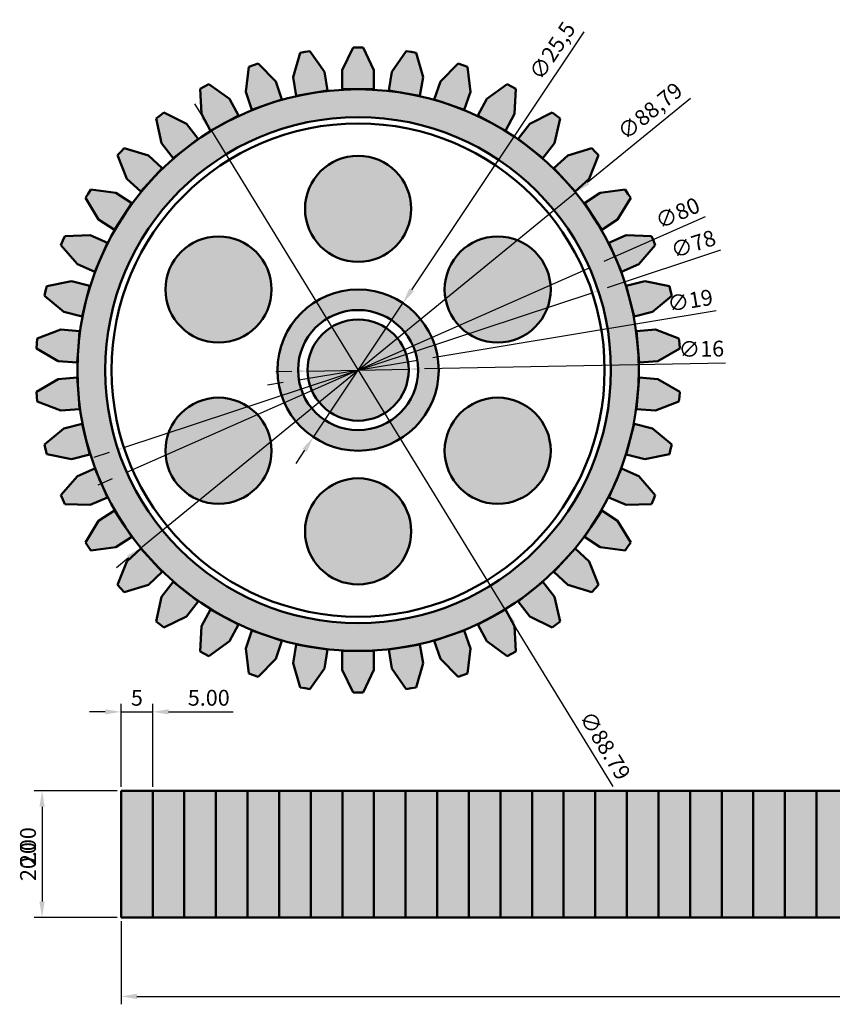
# Model space of a CAD drawing. Units: millimetres. Extents: x 2424 to 2683, y 1522 to 1679.
# Tile 1 of 2: x 2424 to 2552, y 1522 to 1678. Entities that reach past the tile are written whole.
import ezdxf

# ---------------------------------------------------------------- set-up
doc = ezdxf.new("R2010")
doc.units = ezdxf.units.MM
for name, color, linetype, lineweight in [('M-DIMS', 2, 'Continuous', 25), ('M-HATC', 8, 'Continuous', 18), ('M-OUTL', 7, 'Continuous', 50)]:
    doc.layers.add(name, color=color, linetype=linetype, lineweight=lineweight)
doc.styles.get("Standard").update_dxf_attribs({"font": 'arial.ttf'})
doc.dimstyles.new('ISO-25', dxfattribs={"dimtxt": 2.5, "dimasz": 2.5, "dimexe": 1.25, "dimexo": 0.625, "dimtad": 1, "dimtxsty": 'Standard', "dimcen": 2.5, "dimadec": 0, "dimazin": 0, "dimtfac": 1, "dimtmove": 0, "dimatfit": 3, "dimfxl": 1, "dimarcsym": 0})

# ---------------------------------------------------------------- blocks, each defined once
blk = doc.blocks.new('*U1')
for p, q in [((-2.5, -0.3), (-0.78, 3.3)), ((-2.5, -0.3), (-0.78, 3.3)), ((-0.78, 3.3), (0, 3.3)), ((-0.78, 3.3), (0, 3.3)), ((0.78, 3.3), (0, 3.3)), ((0.78, 3.3), (0, 3.3)), ((2.5, -0.3), (0.78, 3.3)), ((2.5, -0.3), (0.78, 3.3)), ((-2.5, -3.3), (-2.5, -0.3)), ((-2.5, -3.3), (-2.5, -0.3)), ((2.5, -3.3), (2.5, -0.3)), ((2.5, -3.3), (2.5, -0.3)), ((0, -3.3), (-2.5, -3.3)), ((0, -3.3), (-2.5, -3.3)), ((0, -3.3), (0, -3.3)), ((0, -3.3), (0, -3.3)), ((0, -3.3), (0, -3.3)), ((0, -3.3), (0, -3.3)), ((0, -3.3), (0, -3.3)), ((0, -3.3), (0, -3.3)), ((0, -3.3), (0, -3.3)), ((0, -3.3), (0, -3.3)), ((0, -3.3), (0, -3.3)), ((0, -3.3), (2.5, -3.3)), ((0, -3.3), (0, -3.3)), ((0, -3.3), (0, -3.3)), ((0, -3.3), (0, -3.3)), ((0, -3.3), (2.5, -3.3))]:
    blk.add_line(p, q)
blk = doc.blocks.new('*U2')
at = {"layer": 'M-OUTL', "color": 0, "linetype": 'ByBlock', "lineweight": -2, "transparency": 16777216}
for p, rotation in [((2469.49, 1669.6), 9.473684210526296), ((2485.19, 1669.6), 350.5263157894737), ((2461.85, 1667.66), 18.94736842105262), ((2492.83, 1667.66), 341.0526315789474), ((2454.64, 1664.5), 28.42105263157894), ((2500.04, 1664.5), 331.578947368421), ((2448.04, 1660.19), 37.89473684210527), ((2506.64, 1660.19), 322.1052631578947), ((2442.25, 1654.85), 47.36842105263155), ((2512.43, 1654.85), 312.6315789473684), ((2437.41, 1648.64), 56.84210526315791), ((2517.27, 1648.64), 303.1578947368421), ((2433.66, 1641.71), 66.31578947368419), ((2521.02, 1641.71), 293.6842105263158), ((2431.1, 1634.26), 75.78947368421053), ((2523.58, 1634.26), 284.2105263157895), ((2429.8, 1626.49), 85.26315789473684), ((2524.87, 1626.49), 274.7368421052631), ((2429.8, 1618.61), 94.73684210526316), ((2524.87, 1618.61), 265.2631578947368), ((2431.1, 1610.84), 104.2105263157894), ((2523.58, 1610.84), 255.7894736842106), ((2433.66, 1603.39), 113.6842105263158), ((2521.02, 1603.39), 246.3157894736842), ((2437.41, 1596.46), 123.1578947368421), ((2517.27, 1596.46), 236.8421052631579), ((2442.25, 1590.24), 132.6315789473684), ((2512.43, 1590.24), 227.3684210526316), ((2448.04, 1584.91), 142.1052631578947), ((2506.64, 1584.91), 217.8947368421053), ((2454.64, 1580.6), 151.578947368421), ((2500.04, 1580.6), 208.4210526315789), ((2461.85, 1577.44), 161.0526315789473), ((2492.83, 1577.44), 198.9473684210526), ((2469.49, 1575.5), 170.5263157894737), ((2485.19, 1575.5), 189.4736842105262), ((2477.34, 1574.85), 180)]:
    blk.add_blockref('*U1', p, dxfattribs=dict(at, rotation=rotation))
blk.add_blockref('*U1', (2477.34, 1670.25), dxfattribs=at)
blk = doc.blocks.new('*U3')
blk.add_circle((0, 0), 8.39)
blk = doc.blocks.new('*U4')
at = {"layer": 'M-OUTL', "color": 0, "linetype": 'ByBlock', "lineweight": -2, "transparency": 16777216}
blk.add_blockref('*U3', (2477.34, 1648.05), dxfattribs=at)
for p, rotation in [((2455.26, 1635.3), 59.99999999999999), ((2499.42, 1635.3), 300), ((2455.26, 1609.8), 120), ((2499.42, 1609.8), 240), ((2477.34, 1597.05), 180)]:
    blk.add_blockref('*U3', p, dxfattribs=dict(at, rotation=rotation))
blk = doc.blocks.new('*D5')
at = {"layer": 'Defpoints', "color": 0, "transparency": 16777216}
for p in [(2511.71, 1650.65), (2442.97, 1594.45)]:
    blk.add_point(p, dxfattribs=at)
at = {"layer": 'M-DIMS', "color": 0, "lineweight": -2, "transparency": 16777216}
for p, q in [((2529.9, 1665.52), (2513.65, 1652.23)), ((2442.97, 1594.45), (2511.71, 1650.65)), ((2441.03, 1592.87), (2439.1, 1591.28))]:
    blk.add_line(p, q, dxfattribs=at)
at = {"layer": 'M-DIMS', "color": 0, "transparency": 16777216}
for points in [[(2513.38, 1652.55), (2513.91, 1651.91), (2511.71, 1650.65)], [(2440.77, 1593.19), (2441.3, 1592.54), (2442.97, 1594.45)]]:
    blk.add_solid(points, dxfattribs=at)
at = {"layer": 'M-DIMS', "color": 0, "transparency": 16777216, "insert": (2523.72, 1663.27), "char_height": 2.5, "attachment_point": 5, "rotation": 39.2675}
blk.add_mtext('∅88,79', dxfattribs=at)
blk = doc.blocks.new('*D6')
at = {"layer": 'Defpoints', "color": 0, "transparency": 16777216}
for p in [(2513.93, 1638.71), (2440.75, 1606.39)]:
    blk.add_point(p, dxfattribs=at)
at = {"layer": 'M-DIMS', "color": 0, "lineweight": -2, "transparency": 16777216}
for p, q in [((2532.26, 1646.81), (2516.22, 1639.72)), ((2440.75, 1606.39), (2513.93, 1638.71)), ((2438.46, 1605.38), (2436.18, 1604.37))]:
    blk.add_line(p, q, dxfattribs=at)
at = {"layer": 'M-DIMS', "color": 0, "transparency": 16777216}
for points in [[(2516.05, 1640.1), (2516.38, 1639.34), (2513.93, 1638.71)], [(2438.29, 1605.76), (2438.63, 1605), (2440.75, 1606.39)]]:
    blk.add_solid(points, dxfattribs=at)
at = {"layer": 'M-DIMS', "color": 0, "transparency": 16777216, "insert": (2528.01, 1647.09), "char_height": 2.5, "attachment_point": 5, "rotation": 23.8315}
blk.add_mtext('∅80', dxfattribs=at)
blk = doc.blocks.new('*D7')
at = {"layer": 'Defpoints', "color": 0, "transparency": 16777216}
for p in [(2514.37, 1634.79), (2440.31, 1610.31)]:
    blk.add_point(p, dxfattribs=at)
at = {"layer": 'M-DIMS', "color": 0, "lineweight": -2, "transparency": 16777216}
for p, q in [((2534.66, 1641.49), (2516.74, 1635.57)), ((2440.31, 1610.31), (2514.37, 1634.79)), ((2437.94, 1609.53), (2435.56, 1608.74))]:
    blk.add_line(p, q, dxfattribs=at)
at = {"layer": 'M-DIMS', "color": 0, "transparency": 16777216}
for points in [[(2516.61, 1635.97), (2516.87, 1635.18), (2514.37, 1634.79)], [(2437.8, 1609.92), (2438.07, 1609.13), (2440.31, 1610.31)]]:
    blk.add_solid(points, dxfattribs=at)
at = {"layer": 'M-DIMS', "color": 0, "transparency": 16777216, "insert": (2530.46, 1642.18), "char_height": 2.5, "attachment_point": 5, "rotation": 18.2866}
blk.add_mtext('∅78', dxfattribs=at)
blk = doc.blocks.new('*D8')
at = {"layer": 'Defpoints', "color": 0, "transparency": 16777216}
for p in [(2484.42, 1633.15), (2470.26, 1611.95)]:
    blk.add_point(p, dxfattribs=at)
at = {"layer": 'M-DIMS', "color": 0, "lineweight": -2, "transparency": 16777216}
for p, q in [((2513.05, 1676.03), (2485.81, 1635.23)), ((2470.26, 1611.95), (2484.42, 1633.15)), ((2468.87, 1609.87), (2467.48, 1607.79))]:
    blk.add_line(p, q, dxfattribs=at)
at = {"layer": 'M-DIMS', "color": 0, "transparency": 16777216}
for points in [[(2485.46, 1635.46), (2486.15, 1635), (2484.42, 1633.15)], [(2468.52, 1610.1), (2469.22, 1609.64), (2470.26, 1611.95)]]:
    blk.add_solid(points, dxfattribs=at)
at = {"layer": 'M-DIMS', "color": 0, "transparency": 16777216, "insert": (2508.33, 1672.87), "char_height": 2.5, "attachment_point": 5, "rotation": 56.2686}
blk.add_mtext('∅25,5', dxfattribs=at)
blk = doc.blocks.new('*D9')
at = {"layer": 'Defpoints', "color": 0, "transparency": 16777216}
for p in [(2486.71, 1624.1), (2467.97, 1621)]:
    blk.add_point(p, dxfattribs=at)
at = {"layer": 'M-DIMS', "color": 0, "lineweight": -2, "transparency": 16777216}
for p, q in [((2533.97, 1631.92), (2489.18, 1624.51)), ((2467.97, 1621), (2486.71, 1624.1)), ((2465.5, 1620.59), (2463.03, 1620.18))]:
    blk.add_line(p, q, dxfattribs=at)
at = {"layer": 'M-DIMS', "color": 0, "transparency": 16777216}
for points in [[(2489.11, 1624.92), (2489.25, 1624.1), (2486.71, 1624.1)], [(2465.43, 1621), (2465.57, 1620.18), (2467.97, 1621)]]:
    blk.add_solid(points, dxfattribs=at)
at = {"layer": 'M-DIMS', "color": 0, "transparency": 16777216, "insert": (2529.92, 1633.24), "char_height": 2.5, "attachment_point": 5, "rotation": 9.3909}
blk.add_mtext('∅19', dxfattribs=at)
blk = doc.blocks.new('*D10')
at = {"layer": 'Defpoints', "color": 0, "transparency": 16777216}
for p in [(2469.34, 1622.39), (2485.34, 1622.7)]:
    blk.add_point(p, dxfattribs=at)
at = {"layer": 'M-DIMS', "color": 0, "lineweight": -2, "transparency": 16777216}
for p, q in [((2466.84, 1622.35), (2464.34, 1622.3)), ((2469.34, 1622.39), (2485.34, 1622.7)), ((2535.46, 1623.67), (2487.84, 1622.75))]:
    blk.add_line(p, q, dxfattribs=at)
at = {"layer": 'M-DIMS', "color": 0, "transparency": 16777216}
for points in [[(2466.83, 1622.76), (2466.85, 1621.93), (2469.34, 1622.39)], [(2487.83, 1623.17), (2487.85, 1622.34), (2485.34, 1622.7)]]:
    blk.add_solid(points, dxfattribs=at)
at = {"layer": 'M-DIMS', "color": 0, "transparency": 16777216, "insert": (2531.64, 1625.57), "char_height": 2.5, "attachment_point": 5, "rotation": 1.1087}
blk.add_mtext('∅16', dxfattribs=at)
blk = doc.blocks.new('*D23')
at = {"layer": 'Defpoints', "color": 0, "transparency": 16777216}
for p in [(2439.85, 1536.01), (2683.5, 1536.01), (2683.5, 1523.51)]:
    blk.add_point(p, dxfattribs=at)
at = {"layer": 'M-DIMS', "color": 0, "lineweight": -2, "transparency": 16777216}
for p, q in [((2439.85, 1535.39), (2439.85, 1522.26)), ((2683.5, 1535.39), (2683.5, 1522.26)), ((2442.35, 1523.51), (2681, 1523.51))]:
    blk.add_line(p, q, dxfattribs=at)
at = {"layer": 'M-DIMS', "color": 0, "transparency": 16777216}
for points in [[(2442.35, 1523.93), (2442.35, 1523.1), (2439.85, 1523.51)], [(2681, 1523.93), (2681, 1523.1), (2683.5, 1523.51)]]:
    blk.add_solid(points, dxfattribs=at)
at = {"layer": 'M-DIMS', "color": 0, "transparency": 16777216, "insert": (2561.68, 1525.41), "char_height": 2.5, "attachment_point": 5}
blk.add_mtext('243.65', dxfattribs=at)
blk = doc.blocks.new('*D24')
at = {"layer": 'Defpoints', "color": 0, "transparency": 16777216}
for p in [(2439.85, 1556.01), (2427.35, 1536.01), (2439.85, 1536.01)]:
    blk.add_point(p, dxfattribs=at)
at = {"layer": 'M-DIMS', "color": 0, "lineweight": -2, "transparency": 16777216}
for p, q in [((2439.23, 1556.01), (2426.1, 1556.01)), ((2427.35, 1553.51), (2427.35, 1538.51)), ((2439.23, 1536.01), (2426.1, 1536.01))]:
    blk.add_line(p, q, dxfattribs=at)
at = {"layer": 'M-DIMS', "color": 0, "transparency": 16777216}
for points in [[(2426.93, 1553.51), (2427.77, 1553.51), (2427.35, 1556.01)], [(2426.93, 1538.51), (2427.77, 1538.51), (2427.35, 1536.01)]]:
    blk.add_solid(points, dxfattribs=at)
at = {"layer": 'M-DIMS', "color": 0, "transparency": 16777216, "insert": (2425.45, 1546.01), "char_height": 2.5, "attachment_point": 5, "rotation": 90}
blk.add_mtext('20', dxfattribs=at)
blk = doc.blocks.new('*D25')
at = {"layer": 'Defpoints', "color": 0, "transparency": 16777216}
for p in [(2444.85, 1568.51), (2439.85, 1556.01), (2444.85, 1556.01)]:
    blk.add_point(p, dxfattribs=at)
at = {"layer": 'M-DIMS', "color": 0, "lineweight": -2, "transparency": 16777216}
for p, q in [((2439.85, 1556.64), (2439.85, 1569.76)), ((2444.85, 1556.64), (2444.85, 1569.76)), ((2437.35, 1568.51), (2434.85, 1568.51)), ((2439.85, 1568.51), (2444.85, 1568.51)), ((2447.35, 1568.51), (2449.85, 1568.51))]:
    blk.add_line(p, q, dxfattribs=at)
at = {"layer": 'M-DIMS', "color": 0, "transparency": 16777216}
for points in [[(2437.35, 1568.93), (2437.35, 1568.1), (2439.85, 1568.51)], [(2447.35, 1568.93), (2447.35, 1568.1), (2444.85, 1568.51)]]:
    blk.add_solid(points, dxfattribs=at)
at = {"layer": 'M-DIMS', "color": 0, "transparency": 16777216, "insert": (2442.35, 1570.41), "char_height": 2.5, "attachment_point": 5}
blk.add_mtext('5', dxfattribs=at)
blk = doc.blocks.new('*D26')
at = {"layer": 'Defpoints', "color": 0, "transparency": 16777216}
for p in [(2439.85, 1536.01), (2683.5, 1536.01), (2683.5, 1523.51)]:
    blk.add_point(p, dxfattribs=at)
at = {"layer": 'M-DIMS', "color": 0, "lineweight": -2, "transparency": 16777216}
for p, q in [((2439.85, 1535.39), (2439.85, 1522.26)), ((2683.5, 1535.39), (2683.5, 1522.26)), ((2442.35, 1523.51), (2681, 1523.51))]:
    blk.add_line(p, q, dxfattribs=at)
at = {"layer": 'M-DIMS', "color": 0, "transparency": 16777216}
for points in [[(2442.35, 1523.93), (2442.35, 1523.1), (2439.85, 1523.51)], [(2681, 1523.93), (2681, 1523.1), (2683.5, 1523.51)]]:
    blk.add_solid(points, dxfattribs=at)
at = {"layer": 'M-DIMS', "color": 0, "transparency": 16777216, "insert": (2561.68, 1525.41), "char_height": 2.5, "attachment_point": 5}
blk.add_mtext('243.65', dxfattribs=at)
blk = doc.blocks.new('*D27')
at = {"layer": 'Defpoints', "color": 0, "transparency": 16777216}
for p in [(2439.85, 1556.01), (2427.35, 1536.01), (2439.85, 1536.01)]:
    blk.add_point(p, dxfattribs=at)
at = {"layer": 'M-DIMS', "color": 0, "lineweight": -2, "transparency": 16777216}
for p, q in [((2439.23, 1556.01), (2426.1, 1556.01)), ((2427.35, 1553.51), (2427.35, 1538.51)), ((2439.23, 1536.01), (2426.1, 1536.01))]:
    blk.add_line(p, q, dxfattribs=at)
at = {"layer": 'M-DIMS', "color": 0, "transparency": 16777216}
for points in [[(2426.93, 1553.51), (2427.77, 1553.51), (2427.35, 1556.01)], [(2426.93, 1538.51), (2427.77, 1538.51), (2427.35, 1536.01)]]:
    blk.add_solid(points, dxfattribs=at)
at = {"layer": 'M-DIMS', "color": 0, "transparency": 16777216, "insert": (2425.45, 1546.01), "char_height": 2.5, "attachment_point": 5, "rotation": 90}
blk.add_mtext('20.00', dxfattribs=at)
blk = doc.blocks.new('*D28')
at = {"layer": 'Defpoints', "color": 0, "transparency": 16777216}
for p in [(2444.85, 1568.51), (2439.85, 1556.01), (2444.85, 1556.01)]:
    blk.add_point(p, dxfattribs=at)
at = {"layer": 'M-DIMS', "color": 0, "lineweight": -2, "transparency": 16777216}
for p, q in [((2439.85, 1556.64), (2439.85, 1569.76)), ((2444.85, 1556.64), (2444.85, 1569.76)), ((2437.35, 1568.51), (2434.85, 1568.51)), ((2439.85, 1568.51), (2444.85, 1568.51)), ((2447.35, 1568.51), (2457.59, 1568.51))]:
    blk.add_line(p, q, dxfattribs=at)
at = {"layer": 'M-DIMS', "color": 0, "transparency": 16777216}
for points in [[(2437.35, 1568.93), (2437.35, 1568.1), (2439.85, 1568.51)], [(2447.35, 1568.93), (2447.35, 1568.1), (2444.85, 1568.51)]]:
    blk.add_solid(points, dxfattribs=at)
at = {"layer": 'M-DIMS', "color": 0, "transparency": 16777216, "insert": (2453.72, 1570.41), "char_height": 2.5, "attachment_point": 5}
blk.add_mtext('5.00', dxfattribs=at)
blk = doc.blocks.new('*D35')
at = {"layer": 'Defpoints', "color": 0, "transparency": 16777216}
for p in [(2454.14, 1660.4), (2500.54, 1584.69)]:
    blk.add_point(p, dxfattribs=at)
at = {"layer": 'M-DIMS', "color": 0, "lineweight": -2, "transparency": 16777216}
for p, q in [((2452.84, 1662.54), (2451.53, 1664.67)), ((2454.14, 1660.4), (2500.54, 1584.69)), ((2517.7, 1556.69), (2501.84, 1582.56))]:
    blk.add_line(p, q, dxfattribs=at)
at = {"layer": 'M-DIMS', "color": 0, "transparency": 16777216}
for points in [[(2453.19, 1662.75), (2452.48, 1662.32), (2454.14, 1660.4)], [(2502.2, 1582.78), (2501.49, 1582.35), (2500.54, 1584.69)]]:
    blk.add_solid(points, dxfattribs=at)
at = {"layer": 'M-DIMS', "color": 0, "transparency": 16777216, "insert": (2516.14, 1563.01), "char_height": 2.5, "attachment_point": 5, "rotation": 301.5003}
blk.add_mtext('∅88.79', dxfattribs=at)

msp = doc.modelspace()

# ---------------------------------------------------------------- hatches: boundary and pattern name
at = {"layer": 'M-HATC'}
h = msp.add_hatch(color=256, dxfattribs=at)
h.set_gradient(color1=(205, 105, 40), color2=(0, 0, 255))
h.paths.add_polyline_path([(2438.3395, 1622.5493, 1), (2516.3395, 1622.5493, 1)], flags=0)
h.paths.add_polyline_path([(2463.6469, 1635.2993, -1), (2446.8649, 1635.2993, -1)], flags=0)
h.paths.add_polyline_path([(2468.9485, 1648.0493, -1), (2485.7305, 1648.0493, -1)], flags=0)
h.paths.add_polyline_path([(2490.0895, 1622.5493, -1), (2464.5895, 1622.5493, -1)], flags=0)
h.paths.add_polyline_path([(2486.8395, 1622.5493, -1), (2467.8395, 1622.5493, -1)], flags=0)
h.paths.add_polyline_path([(2485.3395, 1622.5493, -1), (2469.3395, 1622.5493, -1)], flags=0)
h.paths.add_polyline_path([(2463.6469, 1609.7993, -1), (2446.8649, 1609.7993, -1)], flags=0)
h.paths.add_polyline_path([(2507.8142, 1635.2993, -1), (2491.0322, 1635.2993, -1)], flags=0)
h.paths.add_polyline_path([(2485.7305, 1597.0493, -1), (2468.9485, 1597.0493, -1)], flags=0)
h.paths.add_polyline_path([(2507.8142, 1609.7993, -1), (2491.0322, 1609.7993, -1)], flags=0)
h.paths.add_polyline_path([(2432.9427, 1622.5493, 1), (2521.7364, 1622.5493, 1)])
h.paths.add_polyline_path([(2517.3395, 1622.5493, -1), (2437.3395, 1622.5493, -1)], flags=16)
h.paths.add_polyline_path([(2516.3395, 1622.5493, -1), (2438.3395, 1622.5493, -1)], flags=0)
h.paths.add_polyline_path([(2477.3395, 1666.9462), (2479.8395, 1666.9462), (2479.8395, 1669.9462), (2478.1155, 1673.5434), (2477.3395, 1673.5491), (2476.5636, 1673.5434), (2474.8395, 1669.9462), (2474.8395, 1666.9462)])
h.paths.add_polyline_path([(2484.647, 1666.3407), (2487.1129, 1665.9292), (2487.6067, 1668.8883), (2486.4982, 1672.7202), (2485.7338, 1672.8536), (2484.9675, 1672.9756), (2482.6749, 1669.7112), (2482.1811, 1666.7521)])
h.paths.add_polyline_path([(2494.6312, 1670.5285), (2493.8991, 1670.7858), (2493.1634, 1671.0324), (2490.3647, 1668.1898), (2489.3906, 1665.3524), (2491.7552, 1664.5406), (2494.1197, 1663.7289), (2495.0938, 1666.5663)])
h.paths.add_polyline_path([(2502.2924, 1667.028), (2501.6128, 1667.4023), (2500.9276, 1667.7666), (2497.6992, 1665.4235), (2496.2714, 1662.7851), (2498.4701, 1661.5952), (2500.6688, 1660.4053), (2502.0966, 1663.0437)])
h.paths.add_polyline_path([(2509.2731, 1662.3142), (2508.6643, 1662.7953), (2508.0484, 1663.2674), (2504.4784, 1661.4876), (2502.6358, 1659.1202), (2504.6086, 1657.5847), (2506.5815, 1656.0491), (2508.4241, 1658.4166)], flags=17)
h.paths.add_polyline_path([(2513.9037, 1652.811), (2515.3826, 1656.5158), (2514.8613, 1657.0906), (2514.3316, 1657.6576), (2510.5173, 1656.4896), (2508.3101, 1654.4578), (2510.0033, 1652.6185), (2511.6966, 1650.7792)], flags=0)
h.paths.add_polyline_path([(2520.4545, 1649.7908), (2520.0349, 1650.4436), (2519.6057, 1651.09), (2515.6512, 1650.5659), (2513.1397, 1648.925), (2514.5071, 1646.8321), (2515.8745, 1644.7392), (2518.386, 1646.38)], flags=17)
h.paths.add_polyline_path([(2521.7485, 1639.299), (2524.3502, 1642.3228), (2524.0438, 1643.0357), (2523.7269, 1643.744), (2519.7401, 1643.8779), (2516.9927, 1642.6728), (2517.997, 1640.3833), (2519.0012, 1638.0939)])
h.paths.add_polyline_path([(2523.8998, 1631.7611), (2526.9637, 1634.3154), (2526.7788, 1635.069), (2526.5827, 1635.8198), (2522.6723, 1636.6081), (2519.7641, 1635.8716), (2520.3778, 1633.4481), (2520.9916, 1631.0246)])
h.paths.add_polyline_path([(2521.7912, 1623.7241), (2524.7809, 1623.9719), (2528.2235, 1625.9871), (2528.1652, 1626.7609), (2528.0954, 1627.5337), (2524.368, 1628.9548), (2521.3783, 1628.707), (2521.5847, 1626.2156)])
h.paths.add_polyline_path([(2524.7809, 1621.1268), (2521.7912, 1621.3745), (2521.5847, 1618.8831), (2521.3783, 1616.3916), (2524.368, 1616.1439), (2528.0954, 1617.565), (2528.1652, 1618.3378), (2528.2235, 1619.1116)])
h.paths.add_polyline_path([(2523.8998, 1613.3376), (2520.9916, 1614.074), (2520.3778, 1611.6505), (2519.7641, 1609.227), (2522.6723, 1608.4906), (2526.5827, 1609.2788), (2526.7788, 1610.0296), (2526.9637, 1610.7832)])
h.paths.add_polyline_path([(2521.7485, 1605.7996), (2519.0012, 1607.0047), (2517.997, 1604.7153), (2516.9927, 1602.4259), (2519.7401, 1601.2208), (2523.7269, 1601.3546), (2524.0438, 1602.0629), (2524.3502, 1602.7758)])
h.paths.add_polyline_path([(2518.386, 1598.7186), (2515.8745, 1600.3595), (2514.5071, 1598.2665), (2513.1397, 1596.1736), (2515.6512, 1594.5328), (2519.6057, 1594.0086), (2520.0349, 1594.6551), (2520.4545, 1595.3078)], flags=17)
h.paths.add_polyline_path([(2508.3101, 1590.6408), (2510.5173, 1588.609), (2514.3316, 1587.4411), (2514.8613, 1588.0081), (2515.3826, 1588.5828), (2513.9037, 1592.2876), (2511.6966, 1594.3195), (2510.0033, 1592.4801)], flags=0)
h.paths.add_polyline_path([(2508.4241, 1586.6821), (2506.5815, 1589.0495), (2504.6086, 1587.514), (2502.6358, 1585.9784), (2504.4784, 1583.611), (2508.0484, 1581.8312), (2508.6643, 1582.3033), (2509.2731, 1582.7844)], flags=17)
h.paths.add_polyline_path([(2500.6688, 1584.6933), (2498.4701, 1583.5034), (2496.2714, 1582.3136), (2497.6992, 1579.6752), (2500.9276, 1577.332), (2501.6128, 1577.6963), (2502.2924, 1578.0707), (2502.0966, 1582.0549)])
h.paths.add_polyline_path([(2494.1197, 1581.3698), (2491.7552, 1580.558), (2489.3906, 1579.7463), (2490.3647, 1576.9088), (2493.1634, 1574.0663), (2493.8991, 1574.3128), (2494.6312, 1574.5702), (2495.0938, 1578.5323)])
h.paths.add_polyline_path([(2484.9675, 1572.123), (2485.7338, 1572.2451), (2486.4982, 1572.3784), (2487.6067, 1576.2104), (2487.1129, 1579.1695), (2484.647, 1578.758), (2482.1811, 1578.3465), (2482.6749, 1575.3874)])
h.paths.add_polyline_path([(2479.8395, 1575.1525), (2479.8395, 1578.1525), (2477.3395, 1578.1525), (2474.8395, 1578.1525), (2474.8395, 1575.1525), (2476.5636, 1571.5552), (2477.3395, 1571.5495), (2478.1155, 1571.5552)])
h.paths.add_polyline_path([(2468.1808, 1572.3784), (2468.9452, 1572.2451), (2469.7115, 1572.123), (2472.0042, 1575.3874), (2472.4979, 1578.3465), (2470.032, 1578.758), (2467.5661, 1579.1695), (2467.0723, 1576.2104)])
h.paths.add_polyline_path([(2464.3143, 1576.9088), (2465.2884, 1579.7463), (2462.9239, 1580.558), (2460.5593, 1581.3698), (2459.5852, 1578.5323), (2460.0479, 1574.5702), (2460.7799, 1574.3128), (2461.5157, 1574.0663)])
h.paths.add_polyline_path([(2452.3866, 1578.0707), (2453.0663, 1577.6963), (2453.7514, 1577.332), (2456.9798, 1579.6752), (2458.4076, 1582.3136), (2456.2089, 1583.5034), (2454.0103, 1584.6933), (2452.5824, 1582.0549)])
h.paths.add_polyline_path([(2452.0433, 1585.9784), (2450.0704, 1587.514), (2448.0976, 1589.0495), (2446.2549, 1586.6821), (2445.406, 1582.7844), (2446.0148, 1582.3033), (2446.6306, 1581.8312), (2450.2006, 1583.611)], flags=17)
h.paths.add_polyline_path([(2439.2964, 1588.5828), (2439.8177, 1588.0081), (2440.3475, 1587.4411), (2444.1617, 1588.609), (2446.3689, 1590.6408), (2444.6757, 1592.4801), (2442.9825, 1594.3195), (2440.7753, 1592.2876)], flags=0)
h.paths.add_polyline_path([(2438.8046, 1600.3595), (2436.2931, 1598.7186), (2434.2246, 1595.3078), (2434.6442, 1594.6551), (2435.0734, 1594.0086), (2439.0278, 1594.5328), (2441.5393, 1596.1736), (2440.172, 1598.2665)], flags=17)
h.paths.add_polyline_path([(2436.6821, 1604.7153), (2435.6778, 1607.0047), (2432.9305, 1605.7996), (2430.3288, 1602.7758), (2430.6352, 1602.0629), (2430.9522, 1601.3546), (2434.939, 1601.2208), (2437.6863, 1602.4259)])
h.paths.add_polyline_path([(2432.0067, 1608.4906), (2434.9149, 1609.227), (2434.3012, 1611.6505), (2433.6875, 1614.074), (2430.7793, 1613.3376), (2427.7153, 1610.7832), (2427.9003, 1610.0296), (2428.0963, 1609.2788)])
h.paths.add_polyline_path([(2433.0943, 1618.8831), (2432.8878, 1621.3745), (2429.8981, 1621.1268), (2426.4555, 1619.1116), (2426.5139, 1618.3378), (2426.5837, 1617.565), (2430.311, 1616.1439), (2433.3007, 1616.3916)])
h.paths.add_polyline_path([(2433.0943, 1626.2156), (2433.3007, 1628.707), (2430.311, 1628.9548), (2426.5837, 1627.5337), (2426.5139, 1626.7609), (2426.4555, 1625.9871), (2429.8981, 1623.9719), (2432.8878, 1623.7241)])
h.paths.add_polyline_path([(2430.7793, 1631.7611), (2433.6875, 1631.0246), (2434.3012, 1633.4481), (2434.9149, 1635.8716), (2432.0067, 1636.6081), (2428.0963, 1635.8198), (2427.9003, 1635.069), (2427.7153, 1634.3154)])
h.paths.add_polyline_path([(2435.6778, 1638.0939), (2436.6821, 1640.3833), (2437.6863, 1642.6728), (2434.939, 1643.8779), (2430.9522, 1643.744), (2430.6352, 1643.0357), (2430.3288, 1642.3228), (2432.9305, 1639.299)])
h.paths.add_polyline_path([(2438.8046, 1644.7392), (2440.172, 1646.8321), (2441.5393, 1648.925), (2439.0278, 1650.5659), (2435.0734, 1651.09), (2434.6442, 1650.4436), (2434.2246, 1649.7908), (2436.2931, 1646.38)], flags=17)
h.paths.add_polyline_path([(2444.6757, 1652.6185), (2446.3689, 1654.4578), (2444.1617, 1656.4896), (2440.3475, 1657.6576), (2439.8177, 1657.0906), (2439.2964, 1656.5158), (2440.7753, 1652.811), (2442.9825, 1650.7792)], flags=0)
h.paths.add_polyline_path([(2446.6306, 1663.2674), (2446.0148, 1662.7953), (2445.406, 1662.3142), (2446.2549, 1658.4166), (2448.0976, 1656.0491), (2450.0704, 1657.5847), (2452.0433, 1659.1202), (2450.2006, 1661.4876)], flags=17)
h.paths.add_polyline_path([(2453.7514, 1667.7666), (2453.0663, 1667.4023), (2452.3866, 1667.028), (2452.5824, 1663.0437), (2454.0103, 1660.4053), (2456.2089, 1661.5952), (2458.4076, 1662.7851), (2456.9798, 1665.4235)])
h.paths.add_polyline_path([(2464.3143, 1668.1898), (2461.5157, 1671.0324), (2460.7799, 1670.7858), (2460.0479, 1670.5285), (2459.5852, 1666.5663), (2460.5593, 1663.7289), (2462.9239, 1664.5406), (2465.2884, 1665.3524)])
h.paths.add_polyline_path([(2472.4979, 1666.7521), (2472.0042, 1669.7112), (2469.7115, 1672.9756), (2468.9452, 1672.8536), (2468.1808, 1672.7202), (2467.0723, 1668.8883), (2467.5661, 1665.9292), (2470.032, 1666.3407)])
h = msp.add_hatch(color=256, dxfattribs=at)
h.set_gradient(color1=(255, 0, 0))
h.paths.add_polyline_path([(2444.8516, 1556.0123), (2439.8516, 1556.0123), (2439.8516, 1536.0123), (2444.8516, 1536.0123)])
h.paths.add_polyline_path([(2449.8516, 1556.0123), (2444.8516, 1556.0123), (2444.8516, 1536.0123), (2449.8516, 1536.0123)])
h.paths.add_polyline_path([(2454.8516, 1556.0123), (2449.8516, 1556.0123), (2449.8516, 1536.0123), (2454.8516, 1536.0123)])
h.paths.add_polyline_path([(2459.8516, 1556.0123), (2454.8516, 1556.0123), (2454.8516, 1536.0123), (2459.8516, 1536.0123)])
h.paths.add_polyline_path([(2464.8516, 1556.0123), (2459.8516, 1556.0123), (2459.8516, 1536.0123), (2464.8516, 1536.0123)])
h.paths.add_polyline_path([(2469.8516, 1556.0123), (2464.8516, 1556.0123), (2464.8516, 1536.0123), (2469.8516, 1536.0123)])
h.paths.add_polyline_path([(2474.8516, 1556.0123), (2469.8516, 1556.0123), (2469.8516, 1536.0123), (2474.8516, 1536.0123)])
h.paths.add_polyline_path([(2479.8516, 1556.0123), (2474.8516, 1556.0123), (2474.8516, 1536.0123), (2479.8516, 1536.0123)])
h.paths.add_polyline_path([(2484.8516, 1556.0123), (2479.8516, 1556.0123), (2479.8516, 1536.0123), (2484.8516, 1536.0123)])
h.paths.add_polyline_path([(2489.8516, 1556.0123), (2484.8516, 1556.0123), (2484.8516, 1536.0123), (2489.8516, 1536.0123)])
h.paths.add_polyline_path([(2494.8516, 1556.0123), (2489.8516, 1556.0123), (2489.8516, 1536.0123), (2494.8516, 1536.0123)])
h.paths.add_polyline_path([(2499.8516, 1556.0123), (2494.8516, 1556.0123), (2494.8516, 1536.0123), (2499.8516, 1536.0123)])
h.paths.add_polyline_path([(2504.8516, 1556.0123), (2499.8516, 1556.0123), (2499.8516, 1536.0123), (2504.8516, 1536.0123)])
h.paths.add_polyline_path([(2509.8516, 1556.0123), (2504.8516, 1556.0123), (2504.8516, 1536.0123), (2509.8516, 1536.0123)])
h.paths.add_polyline_path([(2514.8516, 1556.0123), (2509.8516, 1556.0123), (2509.8516, 1536.0123), (2514.8516, 1536.0123)])
h.paths.add_polyline_path([(2519.8516, 1556.0123), (2514.8516, 1556.0123), (2514.8516, 1536.0123), (2519.8516, 1536.0123)])
h.paths.add_polyline_path([(2524.8516, 1556.0123), (2519.8516, 1556.0123), (2519.8516, 1536.0123), (2524.8516, 1536.0123)])
h.paths.add_polyline_path([(2529.8516, 1556.0123), (2524.8516, 1556.0123), (2524.8516, 1536.0123), (2529.8516, 1536.0123)])
h.paths.add_polyline_path([(2534.8516, 1556.0123), (2529.8516, 1556.0123), (2529.8516, 1536.0123), (2534.8516, 1536.0123)])
h.paths.add_polyline_path([(2539.8516, 1556.0123), (2534.8516, 1556.0123), (2534.8516, 1536.0123), (2539.8516, 1536.0123)])
h.paths.add_polyline_path([(2544.8516, 1556.0123), (2539.8516, 1556.0123), (2539.8516, 1536.0123), (2544.8516, 1536.0123)])
h.paths.add_polyline_path([(2549.8516, 1556.0123), (2544.8516, 1556.0123), (2544.8516, 1536.0123), (2549.8516, 1536.0123)])
h.paths.add_polyline_path([(2554.8516, 1556.0123), (2549.8516, 1556.0123), (2549.8516, 1536.0123), (2554.8516, 1536.0123)])
h.paths.add_polyline_path([(2559.8516, 1556.0123), (2554.8516, 1556.0123), (2554.8516, 1536.0123), (2559.8516, 1536.0123)])
h.paths.add_polyline_path([(2564.8516, 1556.0123), (2559.8516, 1556.0123), (2559.8516, 1536.0123), (2564.8516, 1536.0123)])
h.paths.add_polyline_path([(2569.8516, 1556.0123), (2564.8516, 1556.0123), (2564.8516, 1536.0123), (2569.8516, 1536.0123)])
h.paths.add_polyline_path([(2574.8516, 1556.0123), (2569.8516, 1556.0123), (2569.8516, 1536.0123), (2574.8516, 1536.0123)])
h.paths.add_polyline_path([(2579.8516, 1556.0123), (2574.8516, 1556.0123), (2574.8516, 1536.0123), (2579.8516, 1536.0123)])
h.paths.add_polyline_path([(2589.8516, 1556.0123), (2584.8516, 1556.0123), (2584.8516, 1536.0123), (2589.8516, 1536.0123)])
h.paths.add_polyline_path([(2584.8516, 1556.0123), (2579.8516, 1556.0123), (2579.8516, 1536.0123), (2584.8516, 1536.0123)])
h.paths.add_polyline_path([(2594.8516, 1556.0123), (2589.8516, 1556.0123), (2589.8516, 1536.0123), (2594.8516, 1536.0123)])
h.paths.add_polyline_path([(2599.8516, 1556.0123), (2594.8516, 1556.0123), (2594.8516, 1536.0123), (2599.8516, 1536.0123)])
h.paths.add_polyline_path([(2604.8516, 1556.0123), (2599.8516, 1556.0123), (2599.8516, 1536.0123), (2604.8516, 1536.0123)])
h.paths.add_polyline_path([(2609.8516, 1556.0123), (2604.8516, 1556.0123), (2604.8516, 1536.0123), (2609.8516, 1536.0123)])
h.paths.add_polyline_path([(2614.8516, 1556.0123), (2609.8516, 1556.0123), (2609.8516, 1536.0123), (2614.8516, 1536.0123)])
h.paths.add_polyline_path([(2619.8516, 1556.0123), (2614.8516, 1556.0123), (2614.8516, 1536.0123), (2619.8516, 1536.0123)])
h.paths.add_polyline_path([(2624.8516, 1556.0123), (2619.8516, 1556.0123), (2619.8516, 1536.0123), (2624.8516, 1536.0123)])
h.paths.add_polyline_path([(2629.8516, 1556.0123), (2624.8516, 1556.0123), (2624.8516, 1536.0123), (2629.8516, 1536.0123)])
h.paths.add_polyline_path([(2634.8516, 1556.0123), (2629.8516, 1556.0123), (2629.8516, 1536.0123), (2634.8516, 1536.0123)])
h.paths.add_polyline_path([(2639.8516, 1556.0123), (2634.8516, 1556.0123), (2634.8516, 1536.0123), (2639.8516, 1536.0123)])
h.paths.add_polyline_path([(2644.8516, 1556.0123), (2639.8516, 1556.0123), (2639.8516, 1536.0123), (2644.8516, 1536.0123)])
h.paths.add_polyline_path([(2649.8516, 1556.0123), (2644.8516, 1556.0123), (2644.8516, 1536.0123), (2649.8516, 1536.0123)])
h.paths.add_polyline_path([(2654.8516, 1556.0123), (2649.8516, 1556.0123), (2649.8516, 1536.0123), (2654.8516, 1536.0123)])
h.paths.add_polyline_path([(2659.8516, 1556.0123), (2654.8516, 1556.0123), (2654.8516, 1536.0123), (2659.8516, 1536.0123)])
h.paths.add_polyline_path([(2664.8516, 1556.0123), (2659.8516, 1556.0123), (2659.8516, 1536.0123), (2664.8516, 1536.0123)])
h.paths.add_polyline_path([(2669.8516, 1556.0123), (2664.8516, 1556.0123), (2664.8516, 1536.0123), (2669.8516, 1536.0123)])
h.paths.add_polyline_path([(2674.8516, 1556.0123), (2669.8516, 1556.0123), (2669.8516, 1536.0123), (2674.8516, 1536.0123)])
h.paths.add_polyline_path([(2679.8516, 1556.0123), (2674.8516, 1556.0123), (2674.8516, 1536.0123), (2679.8516, 1536.0123)])
h.paths.add_polyline_path([(2683.4993, 1556.0123), (2679.8516, 1556.0123), (2679.8516, 1536.0123), (2683.4993, 1536.0123)])

# ---------------------------------------------------------------- linework, layer by layer
at = {"layer": 'M-OUTL'}
for p, q in [((2477.3395, 1673.5491), (2477.3395, 1673.5493)), ((2439.8516, 1556.0123), (2683.4993, 1556.0123)), ((2439.8516, 1556.0123), (2439.8516, 1536.0123)), ((2439.8516, 1556.0123), (2444.8516, 1556.0123)), ((2444.8516, 1556.0123), (2444.8516, 1536.0123)), ((2449.8516, 1536.0123), (2449.8516, 1556.0123)), ((2454.8516, 1556.0123), (2454.8516, 1536.0123)), ((2459.8516, 1536.0123), (2459.8516, 1556.0123)), ((2464.8516, 1556.0123), (2464.8516, 1536.0123)), ((2469.8516, 1536.0123), (2469.8516, 1556.0123)), ((2474.8516, 1556.0123), (2474.8516, 1536.0123)), ((2479.8516, 1536.0123), (2479.8516, 1556.0123)), ((2484.8516, 1556.0123), (2484.8516, 1536.0123)), ((2489.8516, 1536.0123), (2489.8516, 1556.0123)), ((2494.8516, 1556.0123), (2494.8516, 1536.0123)), ((2499.8516, 1536.0123), (2499.8516, 1556.0123)), ((2504.8516, 1556.0123), (2504.8516, 1536.0123)), ((2509.8516, 1536.0123), (2509.8516, 1556.0123)), ((2514.8516, 1556.0123), (2514.8516, 1536.0123)), ((2519.8516, 1536.0123), (2519.8516, 1556.0123)), ((2524.8516, 1556.0123), (2524.8516, 1536.0123)), ((2529.8516, 1536.0123), (2529.8516, 1556.0123)), ((2534.8516, 1556.0123), (2534.8516, 1536.0123)), ((2539.8516, 1536.0123), (2539.8516, 1556.0123)), ((2544.8516, 1556.0123), (2544.8516, 1536.0123)), ((2549.8516, 1536.0123), (2549.8516, 1556.0123)), ((2683.4993, 1536.0123), (2439.8516, 1536.0123))]:
    msp.add_line(p, q, dxfattribs=at)
for radius in [44.3969, 40, 39, 12.75, 12.75, 9.5, 8]:
    msp.add_circle((2477.3395, 1622.5493), radius, dxfattribs=at)

# ---------------------------------------------------------------- block references
for name in ['*U2', '*U4']:
    msp.add_blockref(name, (0, 0), dxfattribs=at)

# ---------------------------------------------------------------- dimensions: what is measured, and where the dimension line sits
at = {"layer": 'M-DIMS'}
for p1, p2, override, picture, middle in [((2470.2594, 1611.9458), (2484.4196, 1633.1529), {"dimclrd": 0, "dimclre": 0, "dimclrt": 0}, '*D8', (2510.1369, 1671.6687)), ((2442.9675, 1594.4487), (2511.7116, 1650.6499), {"dimclrd": 0, "dimclre": 0, "dimclrt": 0}, '*D5', (2525.0938, 1661.5905)), ((2454.142, 1660.4037), (2500.537, 1584.6949), {"dimdec": 2, "dimlfac": 1, "dimrnd": 0, "dimzin": 0, "dimdsep": 46, "dimlunit": 2}, '*D35', (2514.4555, 1561.9822)), ((2440.75, 1606.3874), (2513.929, 1638.7112), {"dimclrd": 0, "dimclre": 0, "dimclrt": 0}, '*D6', (2528.8103, 1645.2844)), ((2440.3091, 1610.3123), (2514.37, 1634.7864), {"dimclrd": 0, "dimclre": 0, "dimclrt": 0}, '*D7', (2531.0749, 1640.3066)), ((2467.9668, 1620.9992), (2486.7122, 1624.0994), {"dimclrd": 0, "dimclre": 0, "dimclrt": 0}, '*D9', (2530.2436, 1631.2989)), ((2469.341, 1622.3945), (2485.338, 1622.7041), {"dimclrd": 0, "dimclre": 0, "dimclrt": 0}, '*D10', (2531.6811, 1623.601))]:
    dim = msp.add_diameter_dim_2p(p1=p1, p2=p2, dimstyle='ISO-25', override=override, dxfattribs=at)
    dim.commit()
    dim.dimension.update_dxf_attribs({"geometry": picture, "text_midpoint": middle, "dimtype": 163})
for base, p1, p2, override, picture, middle in [((2444.8516, 1568.5123), (2439.8516, 1556.0123), (2444.8516, 1556.0123), {"dimdec": 2, "dimlfac": 1, "dimrnd": 0, "dimzin": 0, "dimdsep": 46, "dimlunit": 2}, '*D28', (2453.7192, 1570.4137)), ((2444.8516, 1568.5123), (2439.8516, 1556.0123), (2444.8516, 1556.0123), {"dimdec": 0, "dimlfac": 1, "dimrnd": 0, "dimzin": 0, "dimdsep": 46, "dimlunit": 2}, '*D25', (2442.3516, 1570.4086)), ((2683.4993, 1523.5123), (2439.8516, 1536.0123), (2683.4993, 1536.0123), {"dimdec": 2, "dimlfac": 1, "dimrnd": 0, "dimzin": 0, "dimdsep": 46, "dimlunit": 2}, '*D23', (2561.6754, 1525.4146)), ((2683.4993, 1523.5123), (2439.8516, 1536.0123), (2683.4993, 1536.0123), {"dimdec": 2, "dimlfac": 1, "dimrnd": 0, "dimzin": 0, "dimdsep": 46, "dimlunit": 2}, '*D26', (2561.6754, 1525.4146))]:
    dim = msp.add_linear_dim(base=base, p1=p1, p2=p2, dimstyle='ISO-25', override=override, dxfattribs=at)
    dim.commit()
    dim.dimension.update_dxf_attribs({"geometry": picture, "text_midpoint": middle})
for override, picture in [({"dimdec": 0, "dimlfac": 1, "dimrnd": 0, "dimzin": 0, "dimdsep": 46, "dimlunit": 2}, '*D24'), ({"dimdec": 2, "dimlfac": 1, "dimrnd": 0, "dimzin": 0, "dimdsep": 46, "dimlunit": 2}, '*D27')]:
    dim = msp.add_linear_dim(base=(2427.3516, 1536.0123), p1=(2439.8516, 1556.0123), p2=(2439.8516, 1536.0123), angle=90, dimstyle='ISO-25', override=override, dxfattribs=at)
    dim.commit()
    dim.dimension.update_dxf_attribs({"geometry": picture, "text_midpoint": (2425.4501, 1546.0123)})

doc.saveas('drawing.dxf')
